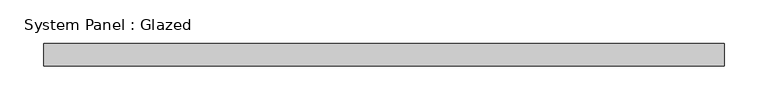
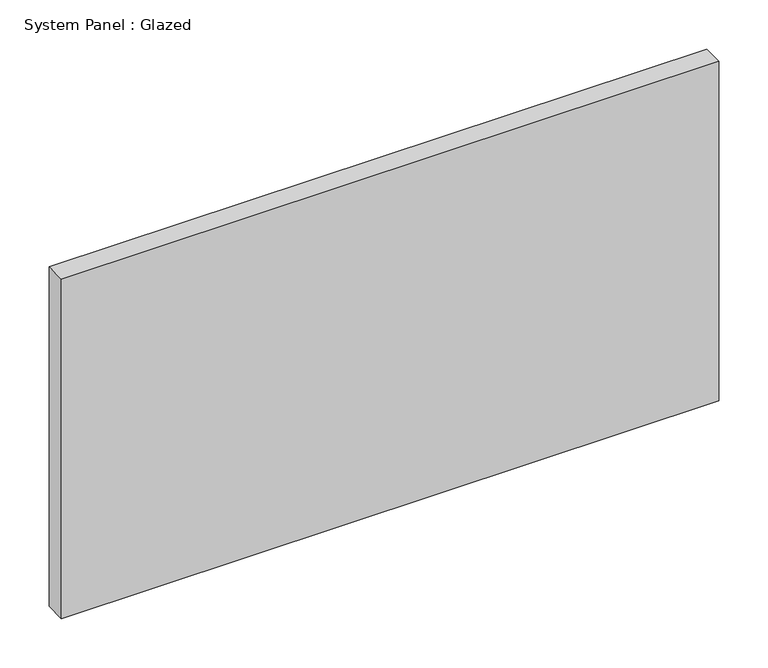
"""IFC4 building model written with IfcOpenShell, lengths in millimetres: plate geometry, System Panel : Glazed."""

from ifc_helpers import new_model, si_unit, origin, origin_with_axes, place, context, project, spatial, polyline, outline, extrude, source, transform, mapped, element, save


def system_panel_glazed_1f22f3a7(model_context):
    return source(origin(), model_context, "Body", "SweptSolid", [
        extrude(outline(polyline([(387.35, 19.05), (-387.35, 19.05), (-387.35, 44.45), (387.35, 44.45), (387.35, 19.05)])), origin_with_axes(), (0.0, 0.0, 1.0), 423.0354569),
    ])


if __name__ == "__main__":
    model = new_model("IFC4")
    model_context = context("Model", 3, world=origin())
    ifc_project = project(units=[si_unit("LENGTHUNIT", "METRE", prefix="MILLI")], contexts=[model_context])
    site = spatial("IfcSite", under=ifc_project)
    building = spatial("IfcBuilding", under=site)
    placement = place(None, origin())
    system_panel_glazed_shape = system_panel_glazed_1f22f3a7(model_context)
    element("IfcPlate", 1, ObjectType="System Panel : Glazed", at=placement, inside=building, context=model_context, shape_type="MappedRepresentation", body=[
        mapped(system_panel_glazed_shape, transform((0.0, 0.0, 0.0), x_axis=(1.0, 0.0, 0.0), y_axis=(0.0, 1.0, 0.0), z_axis=(0.0, 0.0, 1.0))),
    ])
    save(model, "model.ifc")

# Revit data of these elements
# Type "System Panel : Glazed"
#   Construction Type Id = "GSP4R"
#   Analytic Construction = "1/8 in Pilkington single glazing"
#   Visual Light Transmittance = 0.9
#   Solar Heat Gain Coefficient = 0.86
#   Heat Transfer Coefficient (U) = 1.18115 BTU/(h·ft²·°F)
#   Define Thermal Properties by = 1
# Element 1 (IfcPlate, "System Panel : Glazed")
#   Materials on its faces: "Glass"
# Materials
#   "Glass": class "Glass", colour RGB 0 128 192, transparency 0.75, Description = "Soda Lime Glass", Cost = 0
